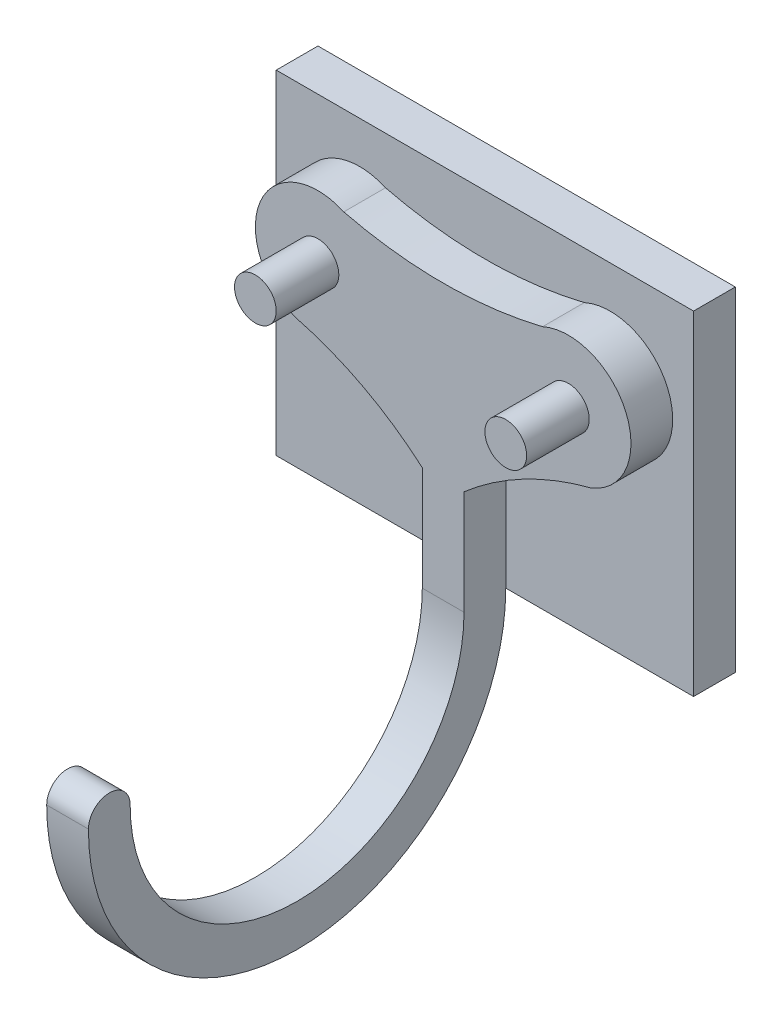
ISO-10303-21;
HEADER;
FILE_DESCRIPTION(('STEP AP214'),'2;1');
FILE_NAME('part.step','',(''),(''),'','','');
FILE_SCHEMA(('AUTOMOTIVE_DESIGN { 1 0 10303 214 1 1 1 1 }'));
ENDSEC;
DATA;
#1=APPLICATION_CONTEXT('core data for automotive mechanical design processes');
#2=APPLICATION_PROTOCOL_DEFINITION('international standard','automotive_design',2000,#1);
#3=PRODUCT_CONTEXT('',#1,'mechanical');
#4=PRODUCT('Part','Part','',(#3));
#5=PRODUCT_RELATED_PRODUCT_CATEGORY('part','',(#4));
#6=PRODUCT_DEFINITION_FORMATION('','',#4);
#7=PRODUCT_DEFINITION_CONTEXT('part definition',#1,'design');
#8=PRODUCT_DEFINITION('design','',#6,#7);
#9=PRODUCT_DEFINITION_SHAPE('','',#8);
#10=(LENGTH_UNIT() NAMED_UNIT(*) SI_UNIT(.MILLI.,.METRE.));
#11=(NAMED_UNIT(*) PLANE_ANGLE_UNIT() SI_UNIT($,.RADIAN.));
#12=(NAMED_UNIT(*) SI_UNIT($,.STERADIAN.) SOLID_ANGLE_UNIT());
#13=UNCERTAINTY_MEASURE_WITH_UNIT(LENGTH_MEASURE(1.E-05),#10,'distance_accuracy_value','');
#14=(GEOMETRIC_REPRESENTATION_CONTEXT(3) GLOBAL_UNCERTAINTY_ASSIGNED_CONTEXT((#13)) GLOBAL_UNIT_ASSIGNED_CONTEXT((#10,
#11,#12)) REPRESENTATION_CONTEXT('',''));
#15=CARTESIAN_POINT('',(0.,0.,0.));
#16=DIRECTION('',(0.,0.,1.));
#17=DIRECTION('',(1.,0.,0.));
#18=AXIS2_PLACEMENT_3D('',#15,#16,#17);
#19=CARTESIAN_POINT('',(-10.,-8.,2.));
#20=DIRECTION('',(0.,1.,0.));
#21=DIRECTION('',(0.,0.,1.));
#22=AXIS2_PLACEMENT_3D('',#19,#20,#21);
#23=PLANE('',#22);
#24=DIRECTION('',(1.,0.,0.));
#25=VECTOR('',#24,1.);
#26=CARTESIAN_POINT('',(-0.999999999999999,-8.,2.));
#27=LINE('',#26,#25);
#28=CARTESIAN_POINT('',(-0.999999999999999,-8.,2.));
#29=VERTEX_POINT('',#28);
#30=CARTESIAN_POINT('',(1.,-8.,2.));
#31=VERTEX_POINT('',#30);
#32=EDGE_CURVE('E143',#29,#31,#27,.T.);
#33=ORIENTED_EDGE('',*,*,#32,.F.);
#34=DIRECTION('',(1.,0.,0.));
#35=VECTOR('',#34,1.);
#36=CARTESIAN_POINT('',(-10.,-8.,2.));
#37=LINE('',#36,#35);
#38=CARTESIAN_POINT('',(-10.,-8.,2.));
#39=VERTEX_POINT('',#38);
#40=EDGE_CURVE('E250',#39,#29,#37,.T.);
#41=ORIENTED_EDGE('',*,*,#40,.F.);
#42=DIRECTION('',(0.,0.,-1.));
#43=VECTOR('',#42,1.);
#44=CARTESIAN_POINT('',(-10.,-8.,2.));
#45=LINE('',#44,#43);
#46=CARTESIAN_POINT('',(-10.,-8.,0.));
#47=VERTEX_POINT('',#46);
#48=EDGE_CURVE('E258',#39,#47,#45,.T.);
#49=ORIENTED_EDGE('',*,*,#48,.T.);
#50=DIRECTION('',(1.,0.,0.));
#51=VECTOR('',#50,1.);
#52=CARTESIAN_POINT('',(-10.,-8.,0.));
#53=LINE('',#52,#51);
#54=CARTESIAN_POINT('',(10.,-8.,0.));
#55=VERTEX_POINT('',#54);
#56=EDGE_CURVE('E245',#47,#55,#53,.T.);
#57=ORIENTED_EDGE('',*,*,#56,.T.);
#58=DIRECTION('',(0.,0.,-1.));
#59=VECTOR('',#58,1.);
#60=CARTESIAN_POINT('',(10.,-8.,2.));
#61=LINE('',#60,#59);
#62=CARTESIAN_POINT('',(10.,-8.,2.));
#63=VERTEX_POINT('',#62);
#64=EDGE_CURVE('E249',#63,#55,#61,.T.);
#65=ORIENTED_EDGE('',*,*,#64,.F.);
#66=EDGE_CURVE('E246',#31,#63,#37,.T.);
#67=ORIENTED_EDGE('',*,*,#66,.F.);
#68=EDGE_LOOP('',(#33,#41,#49,#57,#65,#67));
#69=FACE_BOUND('',#68,.T.);
#70=ADVANCED_FACE('F39',(#69),#23,.F.);
#71=CARTESIAN_POINT('',(10.,-8.,2.));
#72=DIRECTION('',(-1.,0.,0.));
#73=DIRECTION('',(0.,0.,1.));
#74=AXIS2_PLACEMENT_3D('',#71,#72,#73);
#75=PLANE('',#74);
#76=DIRECTION('',(0.,1.,0.));
#77=VECTOR('',#76,1.);
#78=CARTESIAN_POINT('',(10.,-8.,0.));
#79=LINE('',#78,#77);
#80=CARTESIAN_POINT('',(10.,8.,0.));
#81=VERTEX_POINT('',#80);
#82=EDGE_CURVE('E240',#55,#81,#79,.T.);
#83=ORIENTED_EDGE('',*,*,#82,.T.);
#84=DIRECTION('',(0.,0.,-1.));
#85=VECTOR('',#84,1.);
#86=CARTESIAN_POINT('',(10.,8.,2.));
#87=LINE('',#86,#85);
#88=CARTESIAN_POINT('',(10.,8.,2.));
#89=VERTEX_POINT('',#88);
#90=EDGE_CURVE('E11',#89,#81,#87,.T.);
#91=ORIENTED_EDGE('',*,*,#90,.F.);
#92=DIRECTION('',(0.,1.,0.));
#93=VECTOR('',#92,1.);
#94=CARTESIAN_POINT('',(10.,-8.,2.));
#95=LINE('',#94,#93);
#96=EDGE_CURVE('E238',#63,#89,#95,.T.);
#97=ORIENTED_EDGE('',*,*,#96,.F.);
#98=ORIENTED_EDGE('',*,*,#64,.T.);
#99=EDGE_LOOP('',(#83,#91,#97,#98));
#100=FACE_BOUND('',#99,.T.);
#101=ADVANCED_FACE('F41',(#100),#75,.F.);
#102=CARTESIAN_POINT('',(-10.,8.,2.));
#103=DIRECTION('',(0.,-1.,0.));
#104=DIRECTION('',(0.,0.,-1.));
#105=AXIS2_PLACEMENT_3D('',#102,#103,#104);
#106=PLANE('',#105);
#107=DIRECTION('',(-1.,0.,0.));
#108=VECTOR('',#107,1.);
#109=CARTESIAN_POINT('',(-10.,8.,0.));
#110=LINE('',#109,#108);
#111=CARTESIAN_POINT('',(-10.,8.,0.));
#112=VERTEX_POINT('',#111);
#113=EDGE_CURVE('E254',#81,#112,#110,.T.);
#114=ORIENTED_EDGE('',*,*,#113,.T.);
#115=DIRECTION('',(0.,0.,-1.));
#116=VECTOR('',#115,1.);
#117=CARTESIAN_POINT('',(-10.,8.,2.));
#118=LINE('',#117,#116);
#119=CARTESIAN_POINT('',(-10.,8.,2.));
#120=VERTEX_POINT('',#119);
#121=EDGE_CURVE('E50',#120,#112,#118,.T.);
#122=ORIENTED_EDGE('',*,*,#121,.F.);
#123=DIRECTION('',(-1.,0.,0.));
#124=VECTOR('',#123,1.);
#125=CARTESIAN_POINT('',(-10.,8.,2.));
#126=LINE('',#125,#124);
#127=EDGE_CURVE('E241',#89,#120,#126,.T.);
#128=ORIENTED_EDGE('',*,*,#127,.F.);
#129=ORIENTED_EDGE('',*,*,#90,.T.);
#130=EDGE_LOOP('',(#114,#122,#128,#129));
#131=FACE_BOUND('',#130,.T.);
#132=ADVANCED_FACE('F336',(#131),#106,.F.);
#133=CARTESIAN_POINT('',(-10.,-8.,2.));
#134=DIRECTION('',(1.,0.,0.));
#135=DIRECTION('',(0.,0.,-1.));
#136=AXIS2_PLACEMENT_3D('',#133,#134,#135);
#137=PLANE('',#136);
#138=DIRECTION('',(0.,-1.,0.));
#139=VECTOR('',#138,1.);
#140=CARTESIAN_POINT('',(-10.,-8.,0.));
#141=LINE('',#140,#139);
#142=EDGE_CURVE('E253',#112,#47,#141,.T.);
#143=ORIENTED_EDGE('',*,*,#142,.T.);
#144=ORIENTED_EDGE('',*,*,#48,.F.);
#145=DIRECTION('',(0.,-1.,0.));
#146=VECTOR('',#145,1.);
#147=CARTESIAN_POINT('',(-10.,-8.,2.));
#148=LINE('',#147,#146);
#149=EDGE_CURVE('E242',#120,#39,#148,.T.);
#150=ORIENTED_EDGE('',*,*,#149,.F.);
#151=ORIENTED_EDGE('',*,*,#121,.T.);
#152=EDGE_LOOP('',(#143,#144,#150,#151));
#153=FACE_BOUND('',#152,.T.);
#154=ADVANCED_FACE('F270',(#153),#137,.F.);
#155=CARTESIAN_POINT('',(0.,0.,2.));
#156=DIRECTION('',(0.,0.,-1.));
#157=DIRECTION('',(-1.,0.,0.));
#158=AXIS2_PLACEMENT_3D('',#155,#156,#157);
#159=PLANE('',#158);
#160=DIRECTION('',(0.,1.,0.));
#161=VECTOR('',#160,1.);
#162=CARTESIAN_POINT('',(1.,-3.,2.));
#163=LINE('',#162,#161);
#164=CARTESIAN_POINT('',(1.,-3.,2.));
#165=VERTEX_POINT('',#164);
#166=EDGE_CURVE('E216',#31,#165,#163,.T.);
#167=ORIENTED_EDGE('',*,*,#166,.F.);
#168=ORIENTED_EDGE('',*,*,#66,.T.);
#169=ORIENTED_EDGE('',*,*,#96,.T.);
#170=ORIENTED_EDGE('',*,*,#127,.T.);
#171=ORIENTED_EDGE('',*,*,#149,.T.);
#172=ORIENTED_EDGE('',*,*,#40,.T.);
#173=DIRECTION('',(0.,-1.,0.));
#174=VECTOR('',#173,1.);
#175=CARTESIAN_POINT('',(-0.999999999999999,-3.,2.));
#176=LINE('',#175,#174);
#177=CARTESIAN_POINT('',(-1.,-3.,2.));
#178=VERTEX_POINT('',#177);
#179=EDGE_CURVE('E214',#178,#29,#176,.T.);
#180=ORIENTED_EDGE('',*,*,#179,.F.);
#181=CARTESIAN_POINT('',(-10.839043693045,-14.3222444420862,2.));
#182=DIRECTION('',(0.,0.,-1.));
#183=DIRECTION('',(-1.,0.,0.));
#184=AXIS2_PLACEMENT_3D('',#181,#182,#183);
#185=CIRCLE('',#184,15.);
#186=CARTESIAN_POINT('',(-7.06343131978276,0.194805919708031,2.));
#187=VERTEX_POINT('',#186);
#188=EDGE_CURVE('E208',#187,#178,#185,.T.);
#189=ORIENTED_EDGE('',*,*,#188,.F.);
#190=CARTESIAN_POINT('',(-6.,3.,2.));
#191=DIRECTION('',(0.,0.,1.));
#192=DIRECTION('',(1.,0.,0.));
#193=AXIS2_PLACEMENT_3D('',#190,#191,#192);
#194=CIRCLE('',#193,3.);
#195=CARTESIAN_POINT('',(-4.76336301991352,5.73326343031231,2.));
#196=VERTEX_POINT('',#195);
#197=EDGE_CURVE('E210',#196,#187,#194,.T.);
#198=ORIENTED_EDGE('',*,*,#197,.F.);
#199=CARTESIAN_POINT('',(0.,25.157742129637,2.));
#200=DIRECTION('',(0.,0.,-1.));
#201=DIRECTION('',(1.,0.,0.));
#202=AXIS2_PLACEMENT_3D('',#199,#200,#201);
#203=CIRCLE('',#202,20.);
#204=CARTESIAN_POINT('',(4.76336301991352,5.73326343031231,2.));
#205=VERTEX_POINT('',#204);
#206=EDGE_CURVE('E187',#205,#196,#203,.T.);
#207=ORIENTED_EDGE('',*,*,#206,.F.);
#208=CARTESIAN_POINT('',(6.,3.,2.));
#209=DIRECTION('',(0.,0.,1.));
#210=DIRECTION('',(1.,0.,0.));
#211=AXIS2_PLACEMENT_3D('',#208,#209,#210);
#212=CIRCLE('',#211,3.);
#213=CARTESIAN_POINT('',(7.06343131978275,0.19480591970803,2.));
#214=VERTEX_POINT('',#213);
#215=EDGE_CURVE('E56',#214,#205,#212,.T.);
#216=ORIENTED_EDGE('',*,*,#215,.F.);
#217=CARTESIAN_POINT('',(10.839043693045,-14.3222444420862,2.));
#218=DIRECTION('',(0.,0.,-1.));
#219=DIRECTION('',(1.,0.,0.));
#220=AXIS2_PLACEMENT_3D('',#217,#218,#219);
#221=CIRCLE('',#220,15.);
#222=EDGE_CURVE('E53',#165,#214,#221,.T.);
#223=ORIENTED_EDGE('',*,*,#222,.F.);
#224=EDGE_LOOP('',(#167,#168,#169,#170,#171,#172,#180,#189,#198,#207,#216,#223));
#225=FACE_BOUND('',#224,.T.);
#226=ADVANCED_FACE('F278',(#225),#159,.F.);
#227=CARTESIAN_POINT('',(0.,0.,0.));
#228=DIRECTION('',(0.,0.,-1.));
#229=DIRECTION('',(-1.,0.,0.));
#230=AXIS2_PLACEMENT_3D('',#227,#228,#229);
#231=PLANE('',#230);
#232=ORIENTED_EDGE('',*,*,#82,.F.);
#233=ORIENTED_EDGE('',*,*,#56,.F.);
#234=ORIENTED_EDGE('',*,*,#142,.F.);
#235=ORIENTED_EDGE('',*,*,#113,.F.);
#236=EDGE_LOOP('',(#232,#233,#234,#235));
#237=FACE_BOUND('',#236,.T.);
#238=ADVANCED_FACE('F271',(#237),#231,.T.);
#239=CARTESIAN_POINT('',(0.,25.157742129637,4.));
#240=DIRECTION('',(0.,0.,1.));
#241=DIRECTION('',(1.,0.,0.));
#242=AXIS2_PLACEMENT_3D('',#239,#240,#241);
#243=PLANE('',#242);
#244=CARTESIAN_POINT('',(-6.,3.,4.));
#245=DIRECTION('',(0.,0.,1.));
#246=DIRECTION('',(1.,0.,0.));
#247=AXIS2_PLACEMENT_3D('',#244,#245,#246);
#248=CIRCLE('',#247,1.);
#249=CARTESIAN_POINT('',(-5.,3.,4.));
#250=VERTEX_POINT('',#249);
#251=EDGE_CURVE('E182',#250,#250,#248,.T.);
#252=ORIENTED_EDGE('',*,*,#251,.F.);
#253=EDGE_LOOP('',(#252));
#254=FACE_BOUND('',#253,.T.);
#255=CARTESIAN_POINT('',(0.,25.157742129637,4.));
#256=DIRECTION('',(0.,0.,-1.));
#257=DIRECTION('',(1.,0.,0.));
#258=AXIS2_PLACEMENT_3D('',#255,#256,#257);
#259=CIRCLE('',#258,20.);
#260=CARTESIAN_POINT('',(4.76336301991352,5.73326343031231,4.));
#261=VERTEX_POINT('',#260);
#262=CARTESIAN_POINT('',(-4.76336301991352,5.73326343031231,4.));
#263=VERTEX_POINT('',#262);
#264=EDGE_CURVE('E190',#261,#263,#259,.T.);
#265=ORIENTED_EDGE('',*,*,#264,.T.);
#266=CARTESIAN_POINT('',(-6.,3.,4.));
#267=DIRECTION('',(0.,0.,1.));
#268=DIRECTION('',(1.,0.,0.));
#269=AXIS2_PLACEMENT_3D('',#266,#267,#268);
#270=CIRCLE('',#269,3.);
#271=CARTESIAN_POINT('',(-7.06343131978276,0.194805919708031,4.));
#272=VERTEX_POINT('',#271);
#273=EDGE_CURVE('E188',#263,#272,#270,.T.);
#274=ORIENTED_EDGE('',*,*,#273,.T.);
#275=CARTESIAN_POINT('',(-10.839043693045,-14.3222444420862,4.));
#276=DIRECTION('',(0.,0.,-1.));
#277=DIRECTION('',(-1.,0.,0.));
#278=AXIS2_PLACEMENT_3D('',#275,#276,#277);
#279=CIRCLE('',#278,15.);
#280=CARTESIAN_POINT('',(-1.,-3.,4.));
#281=VERTEX_POINT('',#280);
#282=EDGE_CURVE('E195',#272,#281,#279,.T.);
#283=ORIENTED_EDGE('',*,*,#282,.T.);
#284=DIRECTION('',(0.,-1.,0.));
#285=VECTOR('',#284,1.);
#286=CARTESIAN_POINT('',(-0.999999999999999,-3.,4.));
#287=LINE('',#286,#285);
#288=CARTESIAN_POINT('',(-0.999999999999999,-8.,4.));
#289=VERTEX_POINT('',#288);
#290=EDGE_CURVE('E191',#281,#289,#287,.T.);
#291=ORIENTED_EDGE('',*,*,#290,.T.);
#292=DIRECTION('',(1.,0.,0.));
#293=VECTOR('',#292,1.);
#294=CARTESIAN_POINT('',(-0.999999999999999,-8.,4.));
#295=LINE('',#294,#293);
#296=CARTESIAN_POINT('',(1.,-8.,4.));
#297=VERTEX_POINT('',#296);
#298=EDGE_CURVE('E196',#289,#297,#295,.T.);
#299=ORIENTED_EDGE('',*,*,#298,.T.);
#300=DIRECTION('',(0.,1.,0.));
#301=VECTOR('',#300,1.);
#302=CARTESIAN_POINT('',(1.,-3.,4.));
#303=LINE('',#302,#301);
#304=CARTESIAN_POINT('',(1.,-3.,4.));
#305=VERTEX_POINT('',#304);
#306=EDGE_CURVE('E198',#297,#305,#303,.T.);
#307=ORIENTED_EDGE('',*,*,#306,.T.);
#308=CARTESIAN_POINT('',(10.839043693045,-14.3222444420862,4.));
#309=DIRECTION('',(0.,0.,-1.));
#310=DIRECTION('',(1.,0.,0.));
#311=AXIS2_PLACEMENT_3D('',#308,#309,#310);
#312=CIRCLE('',#311,15.);
#313=CARTESIAN_POINT('',(7.06343131978275,0.19480591970803,4.));
#314=VERTEX_POINT('',#313);
#315=EDGE_CURVE('E199',#305,#314,#312,.T.);
#316=ORIENTED_EDGE('',*,*,#315,.T.);
#317=CARTESIAN_POINT('',(6.,3.,4.));
#318=DIRECTION('',(0.,0.,1.));
#319=DIRECTION('',(1.,0.,0.));
#320=AXIS2_PLACEMENT_3D('',#317,#318,#319);
#321=CIRCLE('',#320,3.);
#322=EDGE_CURVE('E205',#314,#261,#321,.T.);
#323=ORIENTED_EDGE('',*,*,#322,.T.);
#324=EDGE_LOOP('',(#265,#274,#283,#291,#299,#307,#316,#323));
#325=FACE_BOUND('',#324,.T.);
#326=CARTESIAN_POINT('',(6.,3.,4.));
#327=DIRECTION('',(0.,0.,1.));
#328=DIRECTION('',(-1.,0.,0.));
#329=AXIS2_PLACEMENT_3D('',#326,#327,#328);
#330=CIRCLE('',#329,1.);
#331=CARTESIAN_POINT('',(5.,3.,4.));
#332=VERTEX_POINT('',#331);
#333=EDGE_CURVE('E179',#332,#332,#330,.T.);
#334=ORIENTED_EDGE('',*,*,#333,.F.);
#335=EDGE_LOOP('',(#334));
#336=FACE_BOUND('',#335,.T.);
#337=ADVANCED_FACE('F307',(#254,#325,#336),#243,.T.);
#338=CARTESIAN_POINT('',(0.,25.157742129637,4.));
#339=DIRECTION('',(0.,0.,-1.));
#340=DIRECTION('',(-1.,0.,0.));
#341=AXIS2_PLACEMENT_3D('',#338,#339,#340);
#342=CYLINDRICAL_SURFACE('',#341,20.);
#343=ORIENTED_EDGE('',*,*,#206,.T.);
#344=DIRECTION('',(0.,0.,-1.));
#345=VECTOR('',#344,1.);
#346=CARTESIAN_POINT('',(-4.76336301991352,5.73326343031231,4.));
#347=LINE('',#346,#345);
#348=EDGE_CURVE('E234',#263,#196,#347,.T.);
#349=ORIENTED_EDGE('',*,*,#348,.F.);
#350=ORIENTED_EDGE('',*,*,#264,.F.);
#351=DIRECTION('',(0.,0.,-1.));
#352=VECTOR('',#351,1.);
#353=CARTESIAN_POINT('',(4.76336301991352,5.73326343031231,4.));
#354=LINE('',#353,#352);
#355=EDGE_CURVE('E201',#261,#205,#354,.T.);
#356=ORIENTED_EDGE('',*,*,#355,.T.);
#357=EDGE_LOOP('',(#343,#349,#350,#356));
#358=FACE_BOUND('',#357,.T.);
#359=ADVANCED_FACE('F294',(#358),#342,.F.);
#360=CARTESIAN_POINT('',(-6.,3.,4.));
#361=DIRECTION('',(0.,0.,-1.));
#362=DIRECTION('',(-1.,0.,0.));
#363=AXIS2_PLACEMENT_3D('',#360,#361,#362);
#364=CYLINDRICAL_SURFACE('',#363,3.);
#365=ORIENTED_EDGE('',*,*,#197,.T.);
#366=DIRECTION('',(0.,0.,-1.));
#367=VECTOR('',#366,1.);
#368=CARTESIAN_POINT('',(-7.06343131978276,0.194805919708031,4.));
#369=LINE('',#368,#367);
#370=EDGE_CURVE('E233',#272,#187,#369,.T.);
#371=ORIENTED_EDGE('',*,*,#370,.F.);
#372=ORIENTED_EDGE('',*,*,#273,.F.);
#373=ORIENTED_EDGE('',*,*,#348,.T.);
#374=EDGE_LOOP('',(#365,#371,#372,#373));
#375=FACE_BOUND('',#374,.T.);
#376=ADVANCED_FACE('F293',(#375),#364,.T.);
#377=CARTESIAN_POINT('',(-10.839043693045,-14.3222444420862,4.));
#378=DIRECTION('',(0.,0.,-1.));
#379=DIRECTION('',(-1.,0.,0.));
#380=AXIS2_PLACEMENT_3D('',#377,#378,#379);
#381=CYLINDRICAL_SURFACE('',#380,15.);
#382=ORIENTED_EDGE('',*,*,#188,.T.);
#383=DIRECTION('',(0.,0.,-1.));
#384=VECTOR('',#383,1.);
#385=CARTESIAN_POINT('',(-1.,-3.,4.));
#386=LINE('',#385,#384);
#387=EDGE_CURVE('E226',#281,#178,#386,.T.);
#388=ORIENTED_EDGE('',*,*,#387,.F.);
#389=ORIENTED_EDGE('',*,*,#282,.F.);
#390=ORIENTED_EDGE('',*,*,#370,.T.);
#391=EDGE_LOOP('',(#382,#388,#389,#390));
#392=FACE_BOUND('',#391,.T.);
#393=ADVANCED_FACE('F289',(#392),#381,.F.);
#394=CARTESIAN_POINT('',(-0.999999999999999,-3.,4.));
#395=DIRECTION('',(1.,0.,0.));
#396=DIRECTION('',(0.,1.,0.));
#397=AXIS2_PLACEMENT_3D('',#394,#395,#396);
#398=PLANE('',#397);
#399=ORIENTED_EDGE('',*,*,#179,.T.);
#400=CARTESIAN_POINT('',(-0.999999999999999,-8.00000000000001,12.));
#401=DIRECTION('',(-1.,0.,0.));
#402=DIRECTION('',(0.,0.,-1.));
#403=AXIS2_PLACEMENT_3D('',#400,#401,#402);
#404=CIRCLE('',#403,10.);
#405=CARTESIAN_POINT('',(-0.999999999999999,-8.00000000000001,22.));
#406=VERTEX_POINT('',#405);
#407=EDGE_CURVE('E156',#29,#406,#404,.T.);
#408=ORIENTED_EDGE('',*,*,#407,.T.);
#409=CARTESIAN_POINT('',(-0.999999999999999,-8.00000000000001,21.));
#410=DIRECTION('',(-1.,0.,0.));
#411=DIRECTION('',(0.,-1.,0.));
#412=AXIS2_PLACEMENT_3D('',#409,#410,#411);
#413=CIRCLE('',#412,0.999999999999999);
#414=CARTESIAN_POINT('',(-0.999999999999999,-8.00000000000001,20.));
#415=VERTEX_POINT('',#414);
#416=EDGE_CURVE('E160',#406,#415,#413,.T.);
#417=ORIENTED_EDGE('',*,*,#416,.T.);
#418=CARTESIAN_POINT('',(-0.999999999999999,-8.00000000000001,12.));
#419=DIRECTION('',(-1.,0.,0.));
#420=DIRECTION('',(0.,0.,-1.));
#421=AXIS2_PLACEMENT_3D('',#418,#419,#420);
#422=CIRCLE('',#421,8.);
#423=EDGE_CURVE('E175',#289,#415,#422,.T.);
#424=ORIENTED_EDGE('',*,*,#423,.F.);
#425=ORIENTED_EDGE('',*,*,#290,.F.);
#426=ORIENTED_EDGE('',*,*,#387,.T.);
#427=EDGE_LOOP('',(#399,#408,#417,#424,#425,#426));
#428=FACE_BOUND('',#427,.T.);
#429=ADVANCED_FACE('F285',(#428),#398,.F.);
#430=CARTESIAN_POINT('',(1.,-3.,4.));
#431=DIRECTION('',(-1.,0.,0.));
#432=DIRECTION('',(0.,-1.,0.));
#433=AXIS2_PLACEMENT_3D('',#430,#431,#432);
#434=PLANE('',#433);
#435=ORIENTED_EDGE('',*,*,#166,.T.);
#436=DIRECTION('',(0.,0.,-1.));
#437=VECTOR('',#436,1.);
#438=CARTESIAN_POINT('',(1.,-3.,4.));
#439=LINE('',#438,#437);
#440=EDGE_CURVE('E223',#305,#165,#439,.T.);
#441=ORIENTED_EDGE('',*,*,#440,.F.);
#442=ORIENTED_EDGE('',*,*,#306,.F.);
#443=CARTESIAN_POINT('',(1.,-8.00000000000001,12.));
#444=DIRECTION('',(-1.,0.,0.));
#445=DIRECTION('',(0.,0.,-1.));
#446=AXIS2_PLACEMENT_3D('',#443,#444,#445);
#447=CIRCLE('',#446,8.);
#448=CARTESIAN_POINT('',(1.,-8.00000000000001,20.));
#449=VERTEX_POINT('',#448);
#450=EDGE_CURVE('E149',#297,#449,#447,.T.);
#451=ORIENTED_EDGE('',*,*,#450,.T.);
#452=CARTESIAN_POINT('',(1.,-8.00000000000001,21.));
#453=DIRECTION('',(-1.,0.,0.));
#454=DIRECTION('',(0.,-1.,0.));
#455=AXIS2_PLACEMENT_3D('',#452,#453,#454);
#456=CIRCLE('',#455,0.999999999999999);
#457=CARTESIAN_POINT('',(1.,-8.00000000000001,22.));
#458=VERTEX_POINT('',#457);
#459=EDGE_CURVE('E154',#458,#449,#456,.T.);
#460=ORIENTED_EDGE('',*,*,#459,.F.);
#461=CARTESIAN_POINT('',(1.,-8.00000000000001,12.));
#462=DIRECTION('',(-1.,0.,0.));
#463=DIRECTION('',(0.,0.,-1.));
#464=AXIS2_PLACEMENT_3D('',#461,#462,#463);
#465=CIRCLE('',#464,10.);
#466=EDGE_CURVE('E136',#31,#458,#465,.T.);
#467=ORIENTED_EDGE('',*,*,#466,.F.);
#468=EDGE_LOOP('',(#435,#441,#442,#451,#460,#467));
#469=FACE_BOUND('',#468,.T.);
#470=ADVANCED_FACE('F162',(#469),#434,.F.);
#471=CARTESIAN_POINT('',(10.839043693045,-14.3222444420862,4.));
#472=DIRECTION('',(0.,0.,-1.));
#473=DIRECTION('',(-1.,0.,0.));
#474=AXIS2_PLACEMENT_3D('',#471,#472,#473);
#475=CYLINDRICAL_SURFACE('',#474,15.);
#476=ORIENTED_EDGE('',*,*,#222,.T.);
#477=DIRECTION('',(0.,0.,-1.));
#478=VECTOR('',#477,1.);
#479=CARTESIAN_POINT('',(7.06343131978275,0.19480591970803,4.));
#480=LINE('',#479,#478);
#481=EDGE_CURVE('E225',#314,#214,#480,.T.);
#482=ORIENTED_EDGE('',*,*,#481,.F.);
#483=ORIENTED_EDGE('',*,*,#315,.F.);
#484=ORIENTED_EDGE('',*,*,#440,.T.);
#485=EDGE_LOOP('',(#476,#482,#483,#484));
#486=FACE_BOUND('',#485,.T.);
#487=ADVANCED_FACE('F303',(#486),#475,.F.);
#488=CARTESIAN_POINT('',(6.,3.,4.));
#489=DIRECTION('',(0.,0.,-1.));
#490=DIRECTION('',(-1.,0.,0.));
#491=AXIS2_PLACEMENT_3D('',#488,#489,#490);
#492=CYLINDRICAL_SURFACE('',#491,3.);
#493=ORIENTED_EDGE('',*,*,#215,.T.);
#494=ORIENTED_EDGE('',*,*,#355,.F.);
#495=ORIENTED_EDGE('',*,*,#322,.F.);
#496=ORIENTED_EDGE('',*,*,#481,.T.);
#497=EDGE_LOOP('',(#493,#494,#495,#496));
#498=FACE_BOUND('',#497,.T.);
#499=ADVANCED_FACE('F296',(#498),#492,.T.);
#500=CARTESIAN_POINT('',(-6.,3.,7.));
#501=DIRECTION('',(0.,0.,-1.));
#502=DIRECTION('',(-1.,0.,0.));
#503=AXIS2_PLACEMENT_3D('',#500,#501,#502);
#504=CYLINDRICAL_SURFACE('',#503,1.);
#505=ORIENTED_EDGE('',*,*,#251,.T.);
#506=EDGE_LOOP('',(#505));
#507=FACE_BOUND('',#506,.T.);
#508=CARTESIAN_POINT('',(-6.,3.,7.));
#509=DIRECTION('',(0.,0.,1.));
#510=DIRECTION('',(1.,0.,0.));
#511=AXIS2_PLACEMENT_3D('',#508,#509,#510);
#512=CIRCLE('',#511,1.);
#513=CARTESIAN_POINT('',(-5.,3.,7.));
#514=VERTEX_POINT('',#513);
#515=EDGE_CURVE('E180',#514,#514,#512,.T.);
#516=ORIENTED_EDGE('',*,*,#515,.F.);
#517=EDGE_LOOP('',(#516));
#518=FACE_BOUND('',#517,.T.);
#519=ADVANCED_FACE('F399',(#507,#518),#504,.T.);
#520=CARTESIAN_POINT('',(-6.,3.,7.));
#521=DIRECTION('',(0.,0.,1.));
#522=DIRECTION('',(1.,0.,0.));
#523=AXIS2_PLACEMENT_3D('',#520,#521,#522);
#524=PLANE('',#523);
#525=ORIENTED_EDGE('',*,*,#515,.T.);
#526=EDGE_LOOP('',(#525));
#527=FACE_BOUND('',#526,.T.);
#528=ADVANCED_FACE('F318',(#527),#524,.T.);
#529=CARTESIAN_POINT('',(6.,3.,7.));
#530=DIRECTION('',(0.,0.,-1.));
#531=DIRECTION('',(-1.,0.,0.));
#532=AXIS2_PLACEMENT_3D('',#529,#530,#531);
#533=CYLINDRICAL_SURFACE('',#532,1.);
#534=ORIENTED_EDGE('',*,*,#333,.T.);
#535=EDGE_LOOP('',(#534));
#536=FACE_BOUND('',#535,.T.);
#537=CARTESIAN_POINT('',(6.,3.,7.));
#538=DIRECTION('',(0.,0.,1.));
#539=DIRECTION('',(1.,0.,0.));
#540=AXIS2_PLACEMENT_3D('',#537,#538,#539);
#541=CIRCLE('',#540,1.);
#542=CARTESIAN_POINT('',(7.,3.,7.));
#543=VERTEX_POINT('',#542);
#544=EDGE_CURVE('E159',#543,#543,#541,.T.);
#545=ORIENTED_EDGE('',*,*,#544,.F.);
#546=EDGE_LOOP('',(#545));
#547=FACE_BOUND('',#546,.T.);
#548=ADVANCED_FACE('F317',(#536,#547),#533,.T.);
#549=CARTESIAN_POINT('',(6.,3.,7.));
#550=DIRECTION('',(0.,0.,1.));
#551=DIRECTION('',(1.,0.,0.));
#552=AXIS2_PLACEMENT_3D('',#549,#550,#551);
#553=PLANE('',#552);
#554=ORIENTED_EDGE('',*,*,#544,.T.);
#555=EDGE_LOOP('',(#554));
#556=FACE_BOUND('',#555,.T.);
#557=ADVANCED_FACE('F316',(#556),#553,.T.);
#558=CARTESIAN_POINT('',(0.,-8.00000000000001,12.));
#559=DIRECTION('',(-1.,0.,0.));
#560=DIRECTION('',(0.,0.,1.));
#561=AXIS2_PLACEMENT_3D('',#558,#559,#560);
#562=CYLINDRICAL_SURFACE('',#561,8.);
#563=ORIENTED_EDGE('',*,*,#423,.T.);
#564=DIRECTION('',(-1.,0.,0.));
#565=VECTOR('',#564,1.);
#566=CARTESIAN_POINT('',(1.,-8.00000000000001,20.));
#567=LINE('',#566,#565);
#568=EDGE_CURVE('E169',#449,#415,#567,.T.);
#569=ORIENTED_EDGE('',*,*,#568,.F.);
#570=ORIENTED_EDGE('',*,*,#450,.F.);
#571=ORIENTED_EDGE('',*,*,#298,.F.);
#572=EDGE_LOOP('',(#563,#569,#570,#571));
#573=FACE_BOUND('',#572,.T.);
#574=ADVANCED_FACE('F308',(#573),#562,.F.);
#575=CARTESIAN_POINT('',(0.,-8.00000000000001,12.));
#576=DIRECTION('',(-1.,0.,0.));
#577=DIRECTION('',(0.,0.,1.));
#578=AXIS2_PLACEMENT_3D('',#575,#576,#577);
#579=CYLINDRICAL_SURFACE('',#578,10.);
#580=DIRECTION('',(1.,0.,0.));
#581=VECTOR('',#580,1.);
#582=CARTESIAN_POINT('',(-0.999999999999999,-8.00000000000001,22.));
#583=LINE('',#582,#581);
#584=EDGE_CURVE('E141',#406,#458,#583,.T.);
#585=ORIENTED_EDGE('',*,*,#584,.F.);
#586=ORIENTED_EDGE('',*,*,#407,.F.);
#587=ORIENTED_EDGE('',*,*,#32,.T.);
#588=ORIENTED_EDGE('',*,*,#466,.T.);
#589=EDGE_LOOP('',(#585,#586,#587,#588));
#590=FACE_BOUND('',#589,.T.);
#591=ADVANCED_FACE('F142',(#590),#579,.T.);
#592=CARTESIAN_POINT('',(1.,-8.00000000000001,21.));
#593=DIRECTION('',(-1.,0.,0.));
#594=DIRECTION('',(0.,-1.,0.));
#595=AXIS2_PLACEMENT_3D('',#592,#593,#594);
#596=CYLINDRICAL_SURFACE('',#595,0.999999999999999);
#597=ORIENTED_EDGE('',*,*,#416,.F.);
#598=ORIENTED_EDGE('',*,*,#584,.T.);
#599=ORIENTED_EDGE('',*,*,#459,.T.);
#600=ORIENTED_EDGE('',*,*,#568,.T.);
#601=EDGE_LOOP('',(#597,#598,#599,#600));
#602=FACE_BOUND('',#601,.T.);
#603=ADVANCED_FACE('F153',(#602),#596,.T.);
#604=CLOSED_SHELL('',(#70,#101,#132,#154,#226,#238,#337,#359,#376,#393,#429,#470,#487,#499,#519,
#528,#548,#557,#574,#591,#603));
#605=MANIFOLD_SOLID_BREP('B2',#604);
#606=ADVANCED_BREP_SHAPE_REPRESENTATION('',(#18,#605),#14);
#607=SHAPE_DEFINITION_REPRESENTATION(#9,#606);
ENDSEC;
END-ISO-10303-21;
